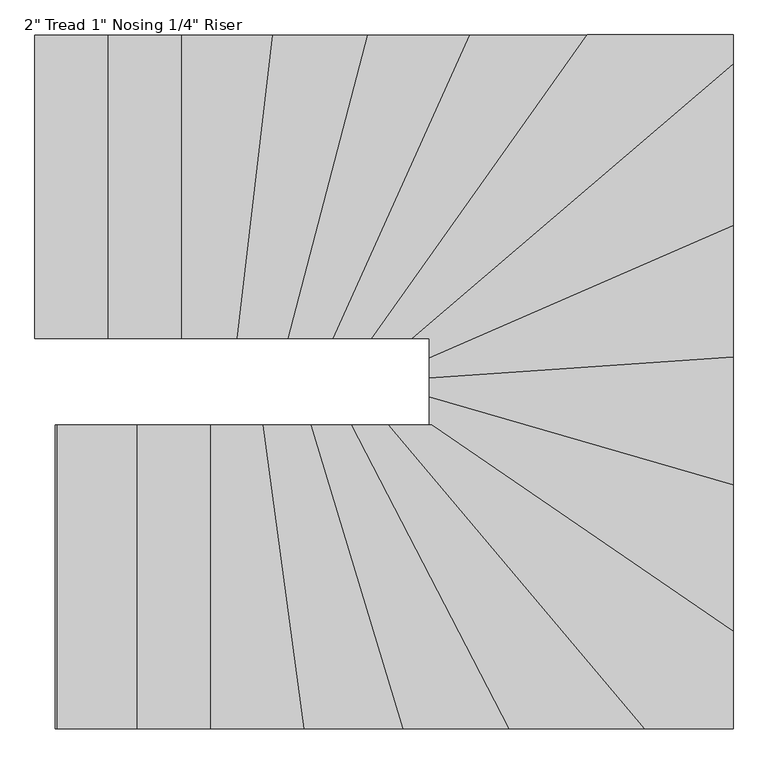
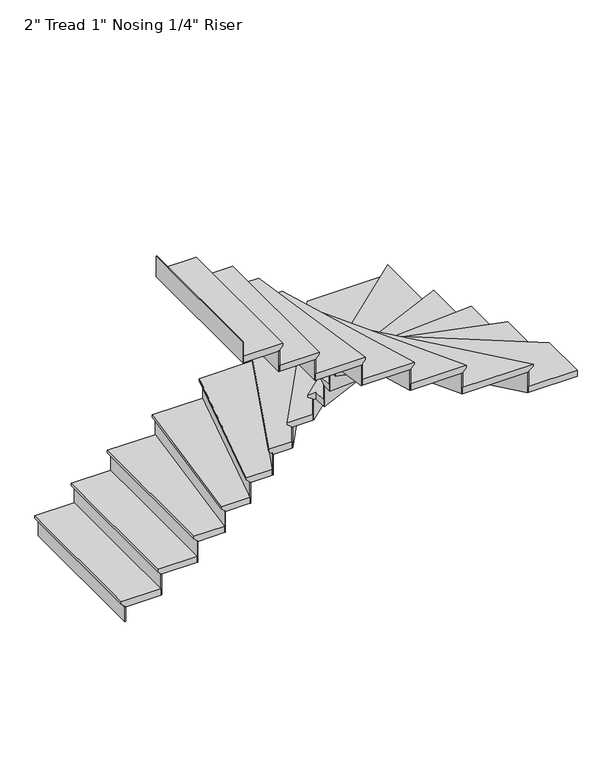
"""IFC4 building model written with IfcOpenShell, lengths in millimetres: stair flight geometry."""

from ifc_helpers import new_model, si_unit, origin, place, context, project, spatial, faceted_brep, source, transform, mapped, element, save


def stair_flight_e7964db3(model_context):
    return source(origin(), model_context, "Body", "Brep", [
        faceted_brep([(-5318.5510787, 1431.1501077, 150.2833333), (-5318.5510787, 1431.1501077, 169.3333333), (-5318.5510787, 2589.1174997, 169.3333333), (-5318.5510787, 2589.1174997, 150.2833333), (-5293.1510787, 1431.1501077, 124.8833333), (-5293.1510787, 2589.1174997, 124.8833333), (-5013.7510787, 1431.1501077, 169.3333333), (-5013.7510787, 2589.1174997, 169.3333333), (-5293.1510787, 2589.1174997, 118.5333333), (-5013.7510787, 2589.1174997, 118.5333333), (-5013.7510787, 1431.1501077, 118.5333333), (-5293.1510787, 1431.1501077, 118.5333333)], [[[0, 1, 2, 3]], [[4, 0, 3, 5]], [[2, 1, 6, 7]], [[8, 9, 10, 11]], [[2, 7, 9, 8, 5, 3]], [[8, 11, 4, 5]], [[6, 1, 0, 4, 11, 10]], [[7, 6, 10, 9]]]),
        faceted_brep([(-5293.1510787, 1431.1501077, 118.5333333), (-5293.1510787, 1431.1501077, 0.0), (-5286.8010787, 1431.1501077, 0.0), (-5286.8010787, 1431.1501077, 118.5333333), (-5293.1510787, 2589.1174997, 118.5333333), (-5286.8010787, 2589.1174997, 118.5333333), (-5286.8010787, 2589.1174997, 0.0), (-5293.1510787, 2589.1174997, 0.0)], [[[0, 1, 2, 3]], [[4, 5, 6, 7]], [[1, 0, 4, 7]], [[2, 1, 7, 6]], [[3, 2, 6, 5]], [[0, 3, 5, 4]]]),
        faceted_brep([(-5013.7510787, 1431.1501077, 287.8666667), (-5013.7510787, 1431.1501077, 118.5333333), (-5007.4010787, 1431.1501077, 118.5333333), (-5007.4010787, 1431.1501077, 287.8666667), (-5013.7510787, 2589.1174997, 287.8666667), (-5007.4010787, 2589.1174997, 287.8666667), (-5007.4010787, 2589.1174997, 118.5333333), (-5013.7510787, 2589.1174997, 118.5333333)], [[[0, 1, 2, 3]], [[4, 5, 6, 7]], [[1, 0, 4, 7]], [[2, 1, 7, 6]], [[3, 2, 6, 5]], [[0, 3, 5, 4]]]),
        faceted_brep([(-5039.1510787, 2589.1174997, 338.6666667), (-5039.1510787, 1431.1501077, 338.6666667), (-4734.3510787, 1431.1501077, 338.6666667), (-4734.3510787, 2589.1174997, 338.6666667), (-5013.7510787, 2589.1174997, 287.8666667), (-4734.3510787, 2589.1174997, 287.8666667), (-4734.3510787, 1431.1501077, 287.8666667), (-5013.7510787, 1431.1501077, 287.8666667), (-5013.7510787, 2589.1174997, 294.2166667), (-5039.1510787, 2589.1174997, 319.6166667), (-5013.7510787, 1431.1501077, 294.2166667), (-5039.1510787, 1431.1501077, 319.6166667)], [[[0, 1, 2, 3]], [[4, 5, 6, 7]], [[0, 3, 5, 4, 8, 9]], [[4, 7, 10, 8]], [[2, 1, 11, 10, 7, 6]], [[3, 2, 6, 5]], [[11, 1, 0, 9]], [[10, 11, 9, 8]]]),
        faceted_brep([(-4734.3510787, 1431.1501077, 457.2), (-4734.3510787, 1431.1501077, 287.8666667), (-4728.0010787, 1431.1501077, 287.8666667), (-4728.0010787, 1431.1501077, 457.2), (-4734.3510787, 2589.1174997, 457.2), (-4728.0010787, 2589.1174997, 457.2), (-4728.0010787, 2589.1174997, 287.8666667), (-4734.3510787, 2589.1174997, 287.8666667)], [[[0, 1, 2, 3]], [[4, 5, 6, 7]], [[1, 0, 4, 7]], [[2, 1, 7, 6]], [[3, 2, 6, 5]], [[0, 3, 5, 4]]]),
        faceted_brep([(-4759.7510787, 2589.1174997, 508.0), (-4759.7510787, 1431.1501077, 508.0), (-4522.1399965, 1431.1501077, 508.0), (-4387.4195146, 2589.1174997, 508.0), (-4734.3510787, 2589.1174997, 457.2), (-4387.4195146, 2589.1174997, 457.2), (-4522.1399965, 1431.1501077, 457.2), (-4734.3510787, 1431.1501077, 457.2), (-4734.3510787, 2589.1174997, 463.55), (-4759.7510787, 2589.1174997, 488.95), (-4734.3510787, 1431.1501077, 463.55), (-4759.7510787, 1431.1501077, 488.95)], [[[0, 1, 2, 3]], [[4, 5, 6, 7]], [[0, 3, 5, 4, 8, 9]], [[4, 7, 10, 8]], [[2, 1, 11, 10, 7, 6]], [[3, 2, 6, 5]], [[11, 1, 0, 9]], [[10, 11, 9, 8]]]),
        faceted_brep([(-4522.1399965, 1431.1501077, 626.5333333), (-4522.1399965, 1431.1501077, 457.2), (-4515.7471657, 1431.1501077, 457.2), (-4515.7471657, 1431.1501077, 626.5333333), (-4387.4195146, 2589.1174997, 626.5333333), (-4381.0266838, 2589.1174997, 626.5333333), (-4381.0266838, 2589.1174997, 457.2), (-4387.4195146, 2589.1174997, 457.2)], [[[0, 1, 2, 3]], [[4, 5, 6, 7]], [[1, 0, 4, 7]], [[2, 1, 7, 6]], [[3, 2, 6, 5]], [[0, 3, 5, 4]]]),
        faceted_brep([(-4412.9908378, 2589.1174997, 677.3333333), (-4547.7113197, 1431.1501077, 677.3333333), (-4326.3090608, 1431.1501077, 677.3333333), (-4023.0802388, 2589.1174997, 677.3333333), (-4387.4195146, 2589.1174997, 626.5333333), (-4023.0802388, 2589.1174997, 626.5333333), (-4326.3090608, 1431.1501077, 626.5333333), (-4522.1399965, 1431.1501077, 626.5333333), (-4387.4195146, 2589.1174997, 632.8833333), (-4412.9908378, 2589.1174997, 658.2833333), (-4522.1399965, 1431.1501077, 632.8833333), (-4547.7113197, 1431.1501077, 658.2833333)], [[[0, 1, 2, 3]], [[4, 5, 6, 7]], [[0, 3, 5, 4, 8, 9]], [[4, 7, 10, 8]], [[2, 1, 11, 10, 7, 6]], [[3, 2, 6, 5]], [[11, 1, 0, 9]], [[10, 11, 9, 8]]]),
        faceted_brep([(-4326.3090608, 1431.1501077, 795.8666667), (-4326.3090608, 1431.1501077, 626.5333333), (-4319.7449535, 1431.1501077, 626.5333333), (-4319.7449535, 1431.1501077, 795.8666667), (-4023.0802388, 2589.1174997, 795.8666667), (-4016.5161315, 2589.1174997, 795.8666667), (-4016.5161315, 2589.1174997, 626.5333333), (-4023.0802388, 2589.1174997, 626.5333333)], [[[0, 1, 2, 3]], [[4, 5, 6, 7]], [[1, 0, 4, 7]], [[2, 1, 7, 6]], [[3, 2, 6, 5]], [[0, 3, 5, 4]]]),
        faceted_brep([(-4049.3366677, 2589.1174997, 846.6666667), (-4352.5654897, 1431.1501077, 846.6666667), (-4153.7362864, 1431.1501077, 846.6666667), (-3633.6777927, 2589.1174997, 846.6666667), (-4023.0802388, 2589.1174997, 795.8666667), (-3633.6777927, 2589.1174997, 795.8666667), (-4153.7362864, 1431.1501077, 795.8666667), (-4326.3090608, 1431.1501077, 795.8666667), (-4023.0802388, 2589.1174997, 802.2166667), (-4049.3366677, 2589.1174997, 827.6166667), (-4326.3090608, 1431.1501077, 802.2166667), (-4352.5654897, 1431.1501077, 827.6166667)], [[[0, 1, 2, 3]], [[4, 5, 6, 7]], [[0, 3, 5, 4, 8, 9]], [[4, 7, 10, 8]], [[2, 1, 11, 10, 7, 6]], [[3, 2, 6, 5]], [[11, 1, 0, 9]], [[10, 11, 9, 8]]]),
        faceted_brep([(-4153.7362864, 1431.1501077, 965.2), (-4153.7362864, 1431.1501077, 795.8666667), (-4146.7752766, 1431.1501077, 795.8666667), (-4146.7752766, 1431.1501077, 965.2), (-3633.6777927, 2589.1174997, 965.2), (-3626.7167829, 2589.1174997, 965.2), (-3626.7167829, 2589.1174997, 795.8666667), (-3633.6777927, 2589.1174997, 795.8666667)], [[[0, 1, 2, 3]], [[4, 5, 6, 7]], [[1, 0, 4, 7]], [[2, 1, 7, 6]], [[3, 2, 6, 5]], [[0, 3, 5, 4]]]),
        faceted_brep([(-3661.5218319, 2589.1174997, 1016.0), (-4181.5803256, 1431.1501077, 1016.0), (-4004.6403592, 1431.1501077, 1016.0), (-3182.5656557, 2589.1174997, 1016.0), (-3633.6777927, 2589.1174997, 965.2), (-3182.5656557, 2589.1174997, 965.2), (-4004.6403592, 1431.1501077, 965.2), (-4153.7362864, 1431.1501077, 965.2), (-3633.6777927, 2589.1174997, 971.55), (-3661.5218319, 2589.1174997, 996.95), (-4153.7362864, 1431.1501077, 971.55), (-4181.5803256, 1431.1501077, 996.95)], [[[0, 1, 2, 3]], [[4, 5, 6, 7]], [[0, 3, 5, 4, 8, 9]], [[4, 7, 10, 8]], [[2, 1, 11, 10, 7, 6]], [[3, 2, 6, 5]], [[11, 1, 0, 9]], [[10, 11, 9, 8]]]),
        faceted_brep([(-4004.6403592, 1431.1501077, 1134.5333333), (-4004.6403592, 1431.1501077, 965.2), (-3996.8528685, 1431.1501077, 965.2), (-3996.8528685, 1431.1501077, 1134.5333333), (-3182.5656557, 2589.1174997, 1134.5333333), (-3174.7781651, 2589.1174997, 1134.5333333), (-3174.7781651, 2589.1174997, 965.2), (-3182.5656557, 2589.1174997, 965.2)], [[[0, 1, 2, 3]], [[4, 5, 6, 7]], [[1, 0, 4, 7]], [[2, 1, 7, 6]], [[3, 2, 6, 5]], [[0, 3, 5, 4]]]),
        faceted_brep([(-2657.7693695, 2444.5732678, 1185.3333333), (-2657.7693695, 2589.1174997, 1185.3333333), (-3213.7156183, 2589.1174997, 1185.3333333), (-4035.7903218, 1431.1501077, 1185.3333333), (-3841.8534644, 1431.1501077, 1185.3333333), (-2657.7693695, 2589.1174997, 1134.5333333), (-2657.7693695, 2444.5732678, 1134.5333333), (-3841.8534644, 1431.1501077, 1134.5333333), (-4004.6403592, 1431.1501077, 1134.5333333), (-3182.5656557, 2589.1174997, 1134.5333333), (-3182.5656557, 2589.1174997, 1140.8833333), (-3213.7156183, 2589.1174997, 1166.2833333), (-4004.6403592, 1431.1501077, 1140.8833333), (-4035.7903218, 1431.1501077, 1166.2833333)], [[[0, 1, 2, 3, 4]], [[5, 6, 7, 8, 9]], [[1, 0, 6, 5]], [[2, 1, 5, 9, 10, 11]], [[9, 8, 12, 10]], [[4, 3, 13, 12, 8, 7]], [[0, 4, 7, 6]], [[13, 3, 2, 11]], [[12, 13, 11, 10]]]),
        faceted_brep([(-3841.8534644, 1431.1501077, 1303.8666667), (-3841.8534644, 1431.1501077, 1134.5333333), (-3832.0877514, 1431.1501077, 1134.5333333), (-3832.0877514, 1431.1501077, 1303.8666667), (-2657.7693695, 2444.5732678, 1303.8666667), (-2657.7693695, 2436.2150779, 1303.8666667), (-2657.7693695, 2436.2150779, 1134.5333333), (-2657.7693695, 2444.5732678, 1134.5333333)], [[[0, 1, 2, 3]], [[4, 5, 6, 7]], [[1, 0, 4, 7]], [[2, 1, 7, 6]], [[3, 2, 6, 5]], [[0, 3, 5, 4]]]),
        faceted_brep([(-2657.7693695, 2478.0060273, 1354.6666667), (-3880.9163163, 1431.1501077, 1354.6666667), (-3815.7367614, 1431.1501077, 1354.6666667), (-3815.7367614, 1329.8462428, 1354.6666667), (-2657.7693695, 1833.9617486, 1354.6666667), (-2657.7693695, 2444.5732678, 1303.8666667), (-2657.7693695, 1833.9617486, 1303.8666667), (-3815.7367614, 1329.8462428, 1303.8666667), (-3815.7367614, 1431.1501077, 1303.8666667), (-3841.8534644, 1431.1501077, 1303.8666667), (-2657.7693695, 2444.5732678, 1310.2166667), (-2657.7693695, 2478.0060273, 1335.6166667), (-3841.8534644, 1431.1501077, 1310.2166667), (-3880.9163163, 1431.1501077, 1335.6166667)], [[[0, 1, 2, 3, 4]], [[5, 6, 7, 8, 9]], [[0, 4, 6, 5, 10, 11]], [[5, 9, 12, 10]], [[3, 2, 8, 7]], [[4, 3, 7, 6]], [[13, 1, 0, 11]], [[12, 13, 11, 10]], [[2, 1, 13, 12, 9, 8]]]),
        faceted_brep([(-3815.7367614, 1329.8462428, 1473.2), (-3815.7367614, 1329.8462428, 1303.8666667), (-3815.7367614, 1322.920592, 1303.8666667), (-3815.7367614, 1322.920592, 1473.2), (-2657.7693695, 1833.9617486, 1473.2), (-2657.7693695, 1827.0360979, 1473.2), (-2657.7693695, 1827.0360979, 1303.8666667), (-2657.7693695, 1833.9617486, 1303.8666667)], [[[0, 1, 2, 3]], [[4, 5, 6, 7]], [[1, 0, 4, 7]], [[2, 1, 7, 6]], [[3, 2, 6, 5]], [[0, 3, 5, 4]]]),
        faceted_brep([(-2657.7693695, 1861.6643517, 1524.0), (-3815.7367614, 1357.5488458, 1524.0), (-3815.7367614, 1254.6233956, 1524.0), (-2657.7693695, 1335.4746165, 1524.0), (-2657.7693695, 1833.9617486, 1473.2), (-2657.7693695, 1335.4746165, 1473.2), (-3815.7367614, 1254.6233956, 1473.2), (-3815.7367614, 1329.8462428, 1473.2), (-2657.7693695, 1833.9617486, 1479.55), (-2657.7693695, 1861.6643517, 1504.95), (-3815.7367614, 1329.8462428, 1479.55), (-3815.7367614, 1357.5488458, 1504.95)], [[[0, 1, 2, 3]], [[4, 5, 6, 7]], [[0, 3, 5, 4, 8, 9]], [[4, 7, 10, 8]], [[2, 1, 11, 10, 7, 6]], [[3, 2, 6, 5]], [[11, 1, 0, 9]], [[10, 11, 9, 8]]]),
        faceted_brep([(-3815.7367614, 1254.6233956, 1642.5333333), (-3815.7367614, 1254.6233956, 1473.2), (-3815.7367614, 1248.2579361, 1473.2), (-3815.7367614, 1248.2579361, 1642.5333333), (-2657.7693695, 1335.4746165, 1642.5333333), (-2657.7693695, 1329.1091569, 1642.5333333), (-2657.7693695, 1329.1091569, 1473.2), (-2657.7693695, 1335.4746165, 1473.2)], [[[0, 1, 2, 3]], [[4, 5, 6, 7]], [[1, 0, 4, 7]], [[2, 1, 7, 6]], [[3, 2, 6, 5]], [[0, 3, 5, 4]]]),
        faceted_brep([(-2657.7693695, 1360.9364545, 1693.3333333), (-3815.7367614, 1280.0852337, 1693.3333333), (-3815.7367614, 1181.6393295, 1693.3333333), (-2657.7693695, 845.9281602, 1693.3333333), (-2657.7693695, 1335.4746165, 1642.5333333), (-2657.7693695, 845.9281602, 1642.5333333), (-3815.7367614, 1181.6393295, 1642.5333333), (-3815.7367614, 1254.6233956, 1642.5333333), (-2657.7693695, 1335.4746165, 1648.8833333), (-2657.7693695, 1360.9364545, 1674.2833333), (-3815.7367614, 1254.6233956, 1648.8833333), (-3815.7367614, 1280.0852337, 1674.2833333)], [[[0, 1, 2, 3]], [[4, 5, 6, 7]], [[0, 3, 5, 4, 8, 9]], [[4, 7, 10, 8]], [[2, 1, 11, 10, 7, 6]], [[3, 2, 6, 5]], [[11, 1, 0, 9]], [[10, 11, 9, 8]]]),
        faceted_brep([(-3815.7367614, 1181.6393295, 1811.8666667), (-3815.7367614, 1181.6393295, 1642.5333333), (-3815.7367614, 1175.0278535, 1642.5333333), (-3815.7367614, 1175.0278535, 1811.8666667), (-2657.7693695, 845.9281602, 1811.8666667), (-2657.7693695, 839.3166841, 1811.8666667), (-2657.7693695, 839.3166841, 1642.5333333), (-2657.7693695, 845.9281602, 1642.5333333)], [[[0, 1, 2, 3]], [[4, 5, 6, 7]], [[1, 0, 4, 7]], [[2, 1, 7, 6]], [[3, 2, 6, 5]], [[0, 3, 5, 4]]]),
        faceted_brep([(-2657.7693695, 872.3740644, 1862.6666667), (-3815.7367614, 1208.0852337, 1862.6666667), (-3815.7367614, 1100.9501077, 1862.6666667), (-3851.4107108, 1100.9501077, 1862.6666667), (-2657.7693695, 284.3923366, 1862.6666667), (-2657.7693695, 845.9281602, 1811.8666667), (-2657.7693695, 284.3923366, 1811.8666667), (-3851.4107108, 1100.9501077, 1811.8666667), (-3815.7367614, 1100.9501077, 1811.8666667), (-3815.7367614, 1181.6393295, 1811.8666667), (-2657.7693695, 845.9281602, 1818.2166667), (-2657.7693695, 872.3740644, 1843.6166667), (-3815.7367614, 1181.6393295, 1818.2166667), (-3815.7367614, 1208.0852337, 1843.6166667)], [[[0, 1, 2, 3, 4]], [[5, 6, 7, 8, 9]], [[0, 4, 6, 5, 10, 11]], [[5, 9, 12, 10]], [[2, 1, 13, 12, 9, 8]], [[4, 3, 7, 6]], [[13, 1, 0, 11]], [[12, 13, 11, 10]], [[3, 2, 8, 7]]]),
        faceted_brep([(-3851.4107108, 1100.9501077, 1981.2), (-3851.4107108, 1100.9501077, 1811.8666667), (-3862.6572925, 1100.9501077, 1811.8666667), (-3862.6572925, 1100.9501077, 1981.2), (-2657.7693695, 284.3923366, 1981.2), (-2657.7693695, 276.6986656, 1981.2), (-2657.7693695, 276.6986656, 1811.8666667), (-2657.7693695, 284.3923366, 1811.8666667)], [[[0, 1, 2, 3]], [[4, 5, 6, 7]], [[1, 0, 4, 7]], [[2, 1, 7, 6]], [[3, 2, 6, 5]], [[0, 3, 5, 4]]]),
        faceted_brep([(-3029.4173018, -57.0172843, 2032.0), (-2657.7693695, -57.0172843, 2032.0), (-2657.7693695, 315.1670204, 2032.0), (-3806.4243837, 1100.9501077, 2032.0), (-4004.9725408, 1100.9501077, 2032.0), (-2657.7693695, -57.0172843, 1981.2), (-3029.4173018, -57.0172843, 1981.2), (-4004.9725408, 1100.9501077, 1981.2), (-3851.4107108, 1100.9501077, 1981.2), (-2657.7693695, 284.3923366, 1981.2), (-3851.4107108, 1100.9501077, 1987.55), (-2657.7693695, 284.3923366, 1987.55), (-3806.4243837, 1100.9501077, 2012.95), (-2657.7693695, 315.1670204, 2012.95)], [[[0, 1, 2, 3, 4]], [[5, 6, 7, 8, 9]], [[1, 0, 6, 5]], [[9, 8, 10, 11]], [[0, 4, 7, 6]], [[12, 3, 2, 13]], [[10, 12, 13, 11]], [[2, 1, 5, 9, 11, 13]], [[4, 3, 12, 10, 8, 7]]]),
        faceted_brep([(-4004.9725408, 1100.9501077, 2150.5333333), (-4004.9725408, 1100.9501077, 1981.2), (-4013.2756588, 1100.9501077, 1981.2), (-4013.2756588, 1100.9501077, 2150.5333333), (-3029.4173018, -57.0172843, 2150.5333333), (-3037.7204198, -57.0172843, 2150.5333333), (-3037.7204198, -57.0172843, 1981.2), (-3029.4173018, -57.0172843, 1981.2)], [[[0, 1, 2, 3]], [[4, 5, 6, 7]], [[1, 0, 4, 7]], [[2, 1, 7, 6]], [[3, 2, 6, 5]], [[0, 3, 5, 4]]]),
        faceted_brep([(-2996.2048299, -57.0172843, 2201.3333333), (-3971.7600689, 1100.9501077, 2201.3333333), (-4142.126531, 1100.9501077, 2201.3333333), (-3540.6187736, -57.0172843, 2201.3333333), (-3029.4173018, -57.0172843, 2150.5333333), (-3540.6187736, -57.0172843, 2150.5333333), (-4142.126531, 1100.9501077, 2150.5333333), (-4004.9725408, 1100.9501077, 2150.5333333), (-3029.4173018, -57.0172843, 2156.8833333), (-2996.2048299, -57.0172843, 2182.2833333), (-4004.9725408, 1100.9501077, 2156.8833333), (-3971.7600689, 1100.9501077, 2182.2833333)], [[[0, 1, 2, 3]], [[4, 5, 6, 7]], [[0, 3, 5, 4, 8, 9]], [[4, 7, 10, 8]], [[2, 1, 11, 10, 7, 6]], [[3, 2, 6, 5]], [[11, 1, 0, 9]], [[10, 11, 9, 8]]]),
        faceted_brep([(-4142.126531, 1100.9501077, 2319.8666667), (-4142.126531, 1100.9501077, 2150.5333333), (-4149.2821378, 1100.9501077, 2150.5333333), (-4149.2821378, 1100.9501077, 2319.8666667), (-3540.6187736, -57.0172843, 2319.8666667), (-3547.7743805, -57.0172843, 2319.8666667), (-3547.7743805, -57.0172843, 2150.5333333), (-3540.6187736, -57.0172843, 2150.5333333)], [[[0, 1, 2, 3]], [[4, 5, 6, 7]], [[1, 0, 4, 7]], [[2, 1, 7, 6]], [[3, 2, 6, 5]], [[0, 3, 5, 4]]]),
        faceted_brep([(-3511.9963462, -57.0172843, 2370.6666667), (-4113.5041036, 1100.9501077, 2370.6666667), (-4294.3324259, 1100.9501077, 2370.6666667), (-3943.0619267, -57.0172843, 2370.6666667), (-3540.6187736, -57.0172843, 2319.8666667), (-3943.0619267, -57.0172843, 2319.8666667), (-4294.3324259, 1100.9501077, 2319.8666667), (-4142.126531, 1100.9501077, 2319.8666667), (-3540.6187736, -57.0172843, 2326.2166667), (-3511.9963462, -57.0172843, 2351.6166667), (-4142.126531, 1100.9501077, 2326.2166667), (-4113.5041036, 1100.9501077, 2351.6166667)], [[[0, 1, 2, 3]], [[4, 5, 6, 7]], [[0, 3, 5, 4, 8, 9]], [[4, 7, 10, 8]], [[2, 1, 11, 10, 7, 6]], [[3, 2, 6, 5]], [[11, 1, 0, 9]], [[10, 11, 9, 8]]]),
        faceted_brep([(-4294.3324259, 1100.9501077, 2489.2), (-4294.3324259, 1100.9501077, 2319.8666667), (-4300.9681662, 1100.9501077, 2319.8666667), (-4300.9681662, 1100.9501077, 2489.2), (-3943.0619267, -57.0172843, 2489.2), (-3949.6976669, -57.0172843, 2489.2), (-3949.6976669, -57.0172843, 2319.8666667), (-3943.0619267, -57.0172843, 2319.8666667)], [[[0, 1, 2, 3]], [[4, 5, 6, 7]], [[1, 0, 4, 7]], [[2, 1, 7, 6]], [[3, 2, 6, 5]], [[0, 3, 5, 4]]]),
        faceted_brep([(-3916.5189656, -57.0172843, 2540.0), (-4267.7894649, 1100.9501077, 2540.0), (-4475.3125347, 1100.9501077, 2540.0), (-4319.0563136, -57.0172843, 2540.0), (-3943.0619267, -57.0172843, 2489.2), (-4319.0563136, -57.0172843, 2489.2), (-4475.3125347, 1100.9501077, 2489.2), (-4294.3324259, 1100.9501077, 2489.2), (-3943.0619267, -57.0172843, 2495.55), (-3916.5189656, -57.0172843, 2520.95), (-4294.3324259, 1100.9501077, 2495.55), (-4267.7894649, 1100.9501077, 2520.95)], [[[0, 1, 2, 3]], [[4, 5, 6, 7]], [[0, 3, 5, 4, 8, 9]], [[4, 7, 10, 8]], [[2, 1, 11, 10, 7, 6]], [[3, 2, 6, 5]], [[11, 1, 0, 9]], [[10, 11, 9, 8]]]),
        faceted_brep([(-4475.3125347, 1100.9501077, 2658.5333333), (-4475.3125347, 1100.9501077, 2489.2), (-4481.7200869, 1100.9501077, 2489.2), (-4481.7200869, 1100.9501077, 2658.5333333), (-4319.0563136, -57.0172843, 2658.5333333), (-4325.4638658, -57.0172843, 2658.5333333), (-4325.4638658, -57.0172843, 2489.2), (-4319.0563136, -57.0172843, 2489.2)], [[[0, 1, 2, 3]], [[4, 5, 6, 7]], [[1, 0, 4, 7]], [[2, 1, 7, 6]], [[3, 2, 6, 5]], [[0, 3, 5, 4]]]),
        faceted_brep([(-4293.4261047, -57.0172843, 2709.3333333), (-4449.6823258, 1100.9501077, 2709.3333333), (-4676.3542153, 1100.9501077, 2709.3333333), (-4676.3542153, -57.0172843, 2709.3333333), (-4319.0563136, -57.0172843, 2658.5333333), (-4676.3542153, -57.0172843, 2658.5333333), (-4676.3542153, 1100.9501077, 2658.5333333), (-4475.3125347, 1100.9501077, 2658.5333333), (-4319.0563136, -57.0172843, 2664.8833333), (-4293.4261047, -57.0172843, 2690.2833333), (-4475.3125347, 1100.9501077, 2664.8833333), (-4449.6823258, 1100.9501077, 2690.2833333)], [[[0, 1, 2, 3]], [[4, 5, 6, 7]], [[0, 3, 5, 4, 8, 9]], [[4, 7, 10, 8]], [[2, 1, 11, 10, 7, 6]], [[3, 2, 6, 5]], [[11, 1, 0, 9]], [[10, 11, 9, 8]]]),
        faceted_brep([(-4676.3542153, 1100.9501077, 2827.8666667), (-4676.3542153, 1100.9501077, 2658.5333333), (-4682.7042153, 1100.9501077, 2658.5333333), (-4682.7042153, 1100.9501077, 2827.8666667), (-4676.3542153, -57.0172843, 2827.8666667), (-4682.7042153, -57.0172843, 2827.8666667), (-4682.7042153, -57.0172843, 2658.5333333), (-4676.3542153, -57.0172843, 2658.5333333)], [[[0, 1, 2, 3]], [[4, 5, 6, 7]], [[1, 0, 4, 7]], [[2, 1, 7, 6]], [[3, 2, 6, 5]], [[0, 3, 5, 4]]]),
        faceted_brep([(-4650.9542153, -57.0172843, 2878.6666667), (-4650.9542153, 1100.9501077, 2878.6666667), (-4955.7542153, 1100.9501077, 2878.6666667), (-4955.7542153, -57.0172843, 2878.6666667), (-4676.3542153, -57.0172843, 2827.8666667), (-4955.7542153, -57.0172843, 2827.8666667), (-4955.7542153, 1100.9501077, 2827.8666667), (-4676.3542153, 1100.9501077, 2827.8666667), (-4676.3542153, -57.0172843, 2834.2166667), (-4650.9542153, -57.0172843, 2859.6166667), (-4676.3542153, 1100.9501077, 2834.2166667), (-4650.9542153, 1100.9501077, 2859.6166667)], [[[0, 1, 2, 3]], [[4, 5, 6, 7]], [[0, 3, 5, 4, 8, 9]], [[4, 7, 10, 8]], [[2, 1, 11, 10, 7, 6]], [[3, 2, 6, 5]], [[11, 1, 0, 9]], [[10, 11, 9, 8]]]),
        faceted_brep([(-4955.7542153, 1100.9501077, 2997.2), (-4955.7542153, 1100.9501077, 2827.8666667), (-4962.1042153, 1100.9501077, 2827.8666667), (-4962.1042153, 1100.9501077, 2997.2), (-4955.7542153, -57.0172843, 2997.2), (-4962.1042153, -57.0172843, 2997.2), (-4962.1042153, -57.0172843, 2827.8666667), (-4955.7542153, -57.0172843, 2827.8666667)], [[[0, 1, 2, 3]], [[4, 5, 6, 7]], [[1, 0, 4, 7]], [[2, 1, 7, 6]], [[3, 2, 6, 5]], [[0, 3, 5, 4]]]),
        faceted_brep([(-5235.1542153, 1100.9501077, 3166.5333333), (-5235.1542153, 1100.9501077, 2997.2), (-5241.5042153, 1100.9501077, 2997.2), (-5241.5042153, 1100.9501077, 3166.5333333), (-5235.1542153, -57.0172843, 3166.5333333), (-5241.5042153, -57.0172843, 3166.5333333), (-5241.5042153, -57.0172843, 2997.2), (-5235.1542153, -57.0172843, 2997.2)], [[[0, 1, 2, 3]], [[4, 5, 6, 7]], [[1, 0, 4, 7]], [[2, 1, 7, 6]], [[3, 2, 6, 5]], [[0, 3, 5, 4]]]),
        faceted_brep([(-4930.3542153, -57.0172843, 3048.0), (-4930.3542153, 1100.9501077, 3048.0), (-5235.1542153, 1100.9501077, 3048.0), (-5235.1542153, -57.0172843, 3048.0), (-4955.7542153, -57.0172843, 2997.2), (-5235.1542153, -57.0172843, 2997.2), (-5235.1542153, 1100.9501077, 2997.2), (-4955.7542153, 1100.9501077, 2997.2), (-4955.7542153, -57.0172843, 3003.55), (-4930.3542153, -57.0172843, 3028.95), (-4955.7542153, 1100.9501077, 3003.55), (-4930.3542153, 1100.9501077, 3028.95)], [[[0, 1, 2, 3]], [[4, 5, 6, 7]], [[0, 3, 5, 4, 8, 9]], [[4, 7, 10, 8]], [[2, 1, 11, 10, 7, 6]], [[3, 2, 6, 5]], [[11, 1, 0, 9]], [[10, 11, 9, 8]]]),
    ])


if __name__ == "__main__":
    model = new_model("IFC4")
    model_context = context("Model", 3, world=origin())
    ifc_project = project(units=[si_unit("LENGTHUNIT", "METRE", prefix="MILLI")], contexts=[model_context])
    site = spatial("IfcSite", under=ifc_project)
    building = spatial("IfcBuilding", under=site)
    placement = place(None, origin())
    stair_flight_shape = stair_flight_e7964db3(model_context)
    element("IfcStairFlight", 1, ObjectType="2\" Tread 1\" Nosing 1/4\" Riser", at=placement, inside=building, context=model_context, shape_type="MappedRepresentation", body=[
        mapped(stair_flight_shape, transform((0.0, 0.0, 0.0), x_axis=(1.0, 0.0, 0.0), y_axis=(0.0, 1.0, 0.0), z_axis=(0.0, 0.0, 1.0))),
    ])
    save(model, "model.ifc")
